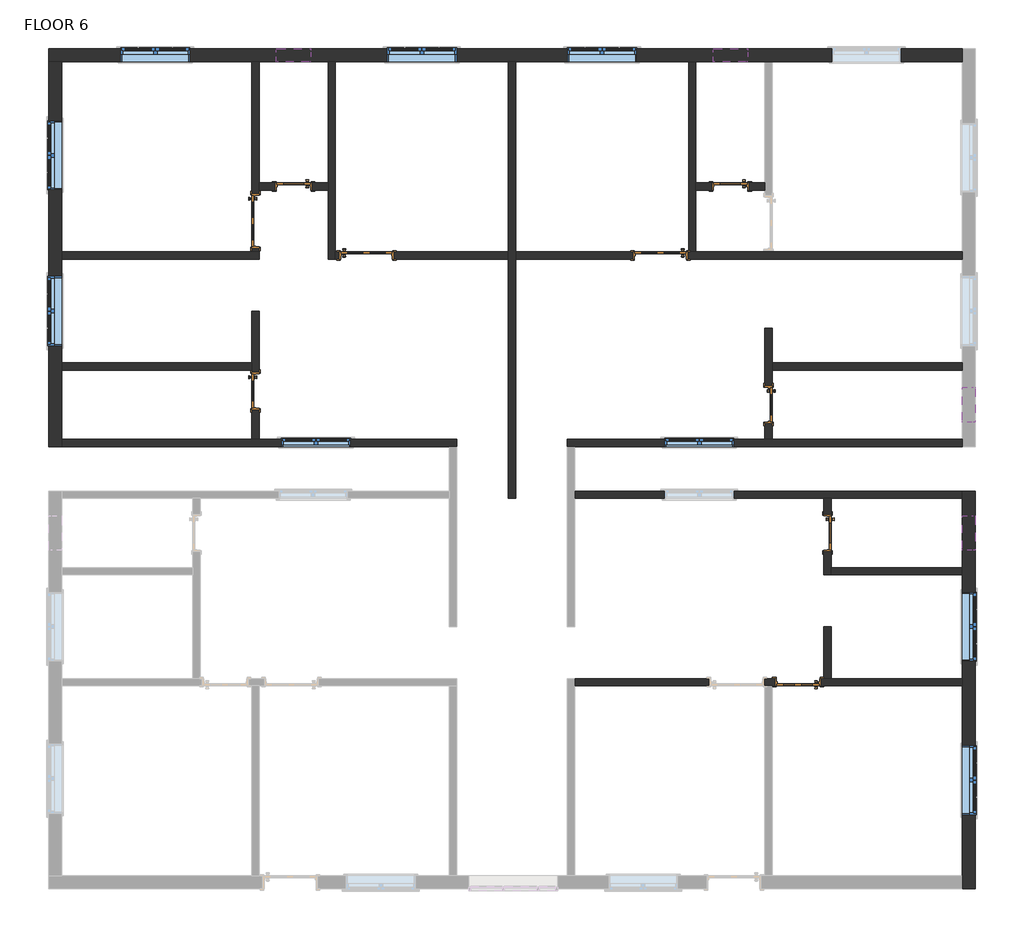
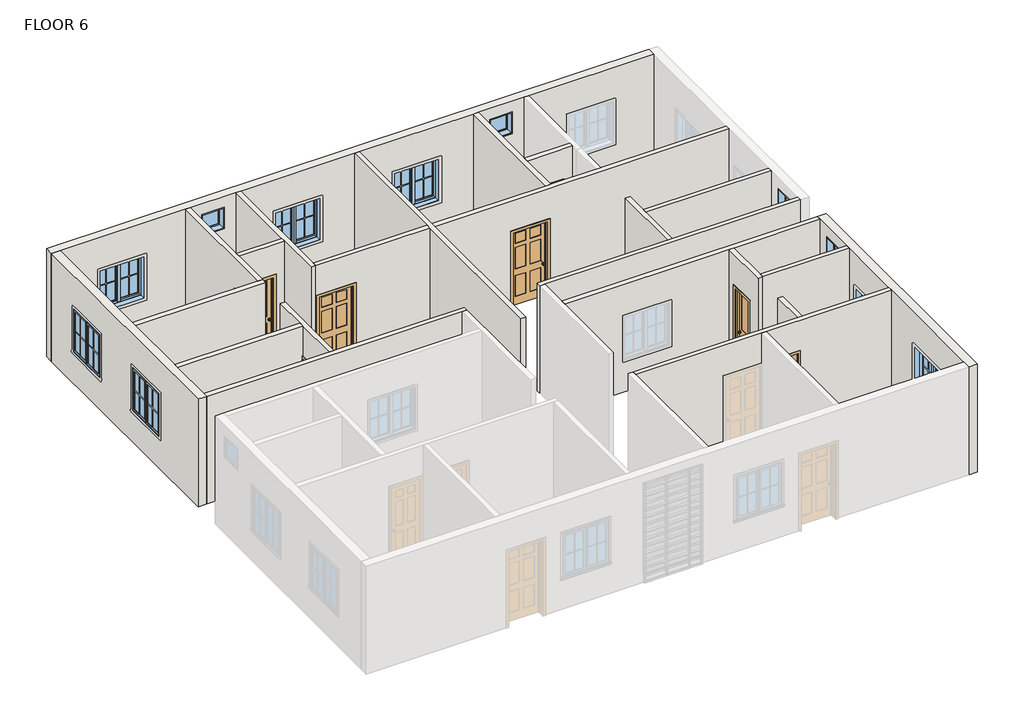
# One storey, part 3 of 4: 23 walls, 13 windows, 9 doors.
"""IFC4 building model written with IfcOpenShell, lengths in millimetres."""

from ifc_helpers import new_model, si_unit, frame, origin, place, context, project, spatial, polyline, outline, extrude, faceted_brep, transform, mapped, element, save
from components import door_e337afa5, door_596d7c92, door_d66ee888, door_c610b25b, door_03e3dfb5, window_80340324, window_9200f5ac, window_c2c97eee

model = new_model("IFC4")

# Units and contexts
model_context = context("Model", 3, world=origin())
ifc_project = project(units=[si_unit("LENGTHUNIT", "METRE", prefix="MILLI")], contexts=[model_context])

# Site, building, storey
site = spatial("IfcSite", under=ifc_project)
building = spatial("IfcBuilding", under=site)
storey = spatial("IfcBuildingStorey", under=building, Name="FLOOR 6", Elevation=9544.3725604)

# Doors
placement = place(None, origin())
door_shape = door_e337afa5(model_context)
element("IfcDoor", 1, ObjectType="Door-Interior-Single-2_Panel-Wood : 24\" x 84\"", at=placement, inside=storey, context=model_context, shape_type="MappedRepresentation", body=[
    mapped(door_shape, transform((-8112.4137331, 4563.2156164, 9544.3725604), x_axis=(-1.0, 0.0, 0.0), y_axis=(0.0, -1.0, 0.0), z_axis=(0.0, 0.0, 1.0))),
])
element("IfcDoor", 2, ObjectType="Door-Interior-Single-2_Panel-Wood : 24\" x 84\"", at=placement, inside=storey, context=model_context, shape_type="MappedRepresentation", body=[
    mapped(door_shape, transform((-416.2137331, 4563.2156164, 9544.3725604), x_axis=(-1.0, 0.0, 0.0), y_axis=(0.0, -1.0, 0.0), z_axis=(0.0, 0.0, 1.0))),
])
element("IfcDoor", 3, ObjectType="Door-Interior-Single-2_Panel-Wood : 24\" x 84\"", at=placement, inside=storey, context=model_context, shape_type="MappedRepresentation", body=[
    mapped(door_shape, transform((-8788.6887331, 953.2406164, 9544.3725604), x_axis=(0.0, -1.0, 0.0), y_axis=(1.0, 0.0, 0.0), z_axis=(0.0, 0.0, 1.0))),
])
door_2_shape = door_596d7c92(model_context)
element("IfcDoor", 4, ObjectType="Door-Interior-Single-2_Panel-Wood : 24\" x 84\"", at=placement, inside=storey, context=model_context, shape_type="MappedRepresentation", body=[
    mapped(door_2_shape, transform((260.0612669, 711.9406164, 9544.3725604), x_axis=(0.0, -1.0, 0.0), y_axis=(1.0, 0.0, 0.0), z_axis=(0.0, 0.0, 1.0))),
])
element("IfcDoor", 5, ObjectType="Door-Interior-Single-2_Panel-Wood : 24\" x 84\"", at=placement, inside=storey, context=model_context, shape_type="MappedRepresentation", body=[
    mapped(door_2_shape, transform((1301.4612669, -1548.6593836, 9544.3725604), x_axis=(0.0, -1.0, 0.0), y_axis=(1.0, 0.0, 0.0), z_axis=(0.0, 0.0, 1.0))),
])
door_3_shape = door_d66ee888(model_context)
element("IfcDoor", 6, ObjectType="Door-Interior-Single-6_Panel-Wood : 30\" x 84\"", at=placement, inside=storey, context=model_context, shape_type="MappedRepresentation", body=[
    mapped(door_3_shape, transform((777.5862669, -4180.7343836, 9544.3725604), x_axis=(-1.0, 0.0, 0.0), y_axis=(0.0, -1.0, 0.0), z_axis=(0.0, 0.0, 1.0))),
])
door_4_shape = door_c610b25b(model_context)
element("IfcDoor", 7, ObjectType="Door-Interior-Single-6_Panel-Wood : 36\" x 84\"", at=placement, inside=storey, context=model_context, shape_type="MappedRepresentation", body=[
    mapped(door_4_shape, transform((-8788.6887331, 3950.4406164, 9544.3725604), x_axis=(0.0, -1.0, 0.0), y_axis=(1.0, 0.0, 0.0), z_axis=(0.0, 0.0, 1.0))),
])
element("IfcDoor", 8, ObjectType="Door-Interior-Single-6_Panel-Wood : 36\" x 84\"", at=placement, inside=storey, context=model_context, shape_type="MappedRepresentation", body=[
    mapped(door_4_shape, transform((-1648.1137331, 3344.0156164, 9544.3725604), x_axis=(-1.0, 0.0, 0.0), y_axis=(0.0, -1.0, 0.0), z_axis=(0.0, 0.0, 1.0))),
])
door_5_shape = door_03e3dfb5(model_context)
element("IfcDoor", 9, ObjectType="Door-Interior-Single-6_Panel-Wood : 36\" x 84\"", at=placement, inside=storey, context=model_context, shape_type="MappedRepresentation", body=[
    mapped(door_5_shape, transform((-6829.7137331, 3344.0156164, 9544.3725604), x_axis=(1.0, 0.0, 0.0), y_axis=(0.0, 1.0, 0.0), z_axis=(0.0, 0.0, 1.0))),
])

# Walls
element("IfcWall", 10, ObjectType="Inner Wall 5\"", at=placement, inside=storey, context=model_context, shape_type="Brep", body=[
    faceted_brep([(-12201.8137331, -24.6593836, 9544.3725604), (-5369.2137331, -24.6593836, 9544.3725604), (-5242.2137331, -24.6593836, 9544.3725604), (-5242.2137331, -24.6593836, 12592.3725604), (-5369.2137331, -24.6593836, 12592.3725604), (-12201.8137331, -24.6593836, 12592.3725604), (-7109.1137331, -24.6593836, 11677.9725604), (-7109.1137331, -24.6593836, 10458.7725604), (-8328.3137331, -24.6593836, 10458.7725604), (-8328.3137331, -24.6593836, 11677.9725604), (-12201.8137331, 102.3406164, 9544.3725604), (-12201.8137331, 102.3406164, 12592.3725604), (-8849.0137331, 102.3406164, 12592.3725604), (-8722.0137331, 102.3406164, 12592.3725604), (-5242.2137331, 102.3406164, 12592.3725604), (-5242.2137331, 102.3406164, 9544.3725604), (-8722.0137331, 102.3406164, 9544.3725604), (-8849.0137331, 102.3406164, 9544.3725604), (-7109.1137331, 102.3406164, 11677.9725604), (-8328.3137331, 102.3406164, 11677.9725604), (-8328.3137331, 102.3406164, 10458.7725604), (-7109.1137331, 102.3406164, 10458.7725604)], [[[0, 1, 2, 3, 4, 5], [6, 7, 8, 9]], [[10, 11, 12, 13, 14, 15, 16, 17], [18, 19, 20, 21]], [[2, 1, 0, 10, 17, 16, 15]], [[5, 4, 3, 14, 13, 12, 11]], [[0, 5, 11, 10]], [[3, 2, 15, 14]], [[7, 6, 18, 21]], [[8, 7, 21, 20]], [[9, 8, 20, 19]], [[6, 9, 19, 18]]]),
])
element("IfcWall", 11, ObjectType="Inner Wall 5\"", at=placement, inside=storey, context=model_context, shape_type="Brep", body=[
    faceted_brep([(3673.1862669, 102.3406164, 9544.3725604), (320.3862669, 102.3406164, 9544.3725604), (193.3862669, 102.3406164, 9544.3725604), (-3286.4137331, 102.3406164, 9544.3725604), (-3286.4137331, 102.3406164, 12592.3725604), (193.3862669, 102.3406164, 12592.3725604), (320.3862669, 102.3406164, 12592.3725604), (3673.1862669, 102.3406164, 12592.3725604), (-352.7137331, 102.3406164, 11677.9725604), (-1571.9137331, 102.3406164, 11677.9725604), (-1571.9137331, 102.3406164, 10458.7725604), (-352.7137331, 102.3406164, 10458.7725604), (3673.1862669, -24.6593836, 9544.3725604), (3673.1862669, -24.6593836, 12592.3725604), (-3159.4137331, -24.6593836, 12592.3725604), (-3286.4137331, -24.6593836, 12592.3725604), (-3286.4137331, -24.6593836, 9544.3725604), (-3159.4137331, -24.6593836, 9544.3725604), (-352.7137331, -24.6593836, 11677.9725604), (-352.7137331, -24.6593836, 10458.7725604), (-1571.9137331, -24.6593836, 10458.7725604), (-1571.9137331, -24.6593836, 11677.9725604)], [[[0, 1, 2, 3, 4, 5, 6, 7], [8, 9, 10, 11]], [[12, 13, 14, 15, 16, 17], [18, 19, 20, 21]], [[3, 2, 1, 0, 12, 17, 16]], [[7, 6, 5, 4, 15, 14, 13]], [[0, 7, 13, 12]], [[4, 3, 16, 15]], [[19, 18, 8, 11]], [[20, 19, 11, 10]], [[21, 20, 10, 9]], [[18, 21, 9, 8]]]),
])
element("IfcWall", 12, ObjectType="Inner Wall 5\"", at=placement, inside=storey, context=model_context, shape_type="Brep", body=[
    faceted_brep([(3673.1862669, -812.0593836, 9544.3725604), (-3159.4137331, -812.0593836, 9544.3725604), (-3159.4137331, -812.0593836, 12592.3725604), (3673.1862669, -812.0593836, 12592.3725604), (-352.7137331, -812.0593836, 11677.9725604), (-1571.9137331, -812.0593836, 11677.9725604), (-1571.9137331, -812.0593836, 10458.7725604), (-352.7137331, -812.0593836, 10458.7725604), (3673.1862669, -939.0593836, 9544.3725604), (3673.1862669, -939.0593836, 12592.3725604), (1361.7862669, -939.0593836, 12592.3725604), (1234.7862669, -939.0593836, 12592.3725604), (-3159.4137331, -939.0593836, 12592.3725604), (-3159.4137331, -939.0593836, 9544.3725604), (1234.7862669, -939.0593836, 9544.3725604), (1361.7862669, -939.0593836, 9544.3725604), (-352.7137331, -939.0593836, 11677.9725604), (-352.7137331, -939.0593836, 10458.7725604), (-1571.9137331, -939.0593836, 10458.7725604), (-1571.9137331, -939.0593836, 11677.9725604)], [[[0, 1, 2, 3], [4, 5, 6, 7]], [[8, 9, 10, 11, 12, 13, 14, 15], [16, 17, 18, 19]], [[1, 0, 8, 15, 14, 13]], [[3, 2, 12, 11, 10, 9]], [[0, 3, 9, 8]], [[2, 1, 13, 12]], [[17, 16, 4, 7]], [[18, 17, 7, 6]], [[19, 18, 6, 5]], [[16, 19, 5, 4]]]),
])
element("IfcWall", 13, ObjectType="Inner Wall 5\"", at=placement, inside=storey, context=model_context, shape_type="Brep", body=[
    faceted_brep([(1234.7862669, -2285.2593836, 12592.3725604), (1234.7862669, -939.0593836, 12592.3725604), (1234.7862669, -939.0593836, 9544.3725604), (1234.7862669, -1218.4593836, 9544.3725604), (1234.7862669, -1218.4593836, 11703.3725604), (1234.7862669, -1878.8593836, 11703.3725604), (1234.7862669, -1878.8593836, 9544.3725604), (1234.7862669, -2285.2593836, 9544.3725604), (1361.7862669, -939.0593836, 12592.3725604), (1361.7862669, -2158.2593836, 12592.3725604), (1361.7862669, -2285.2593836, 12592.3725604), (1361.7862669, -2285.2593836, 9544.3725604), (1361.7862669, -2158.2593836, 9544.3725604), (1361.7862669, -1878.8593836, 9544.3725604), (1361.7862669, -1878.8593836, 11703.3725604), (1361.7862669, -1218.4593836, 11703.3725604), (1361.7862669, -1218.4593836, 9544.3725604), (1361.7862669, -939.0593836, 9544.3725604)], [[[0, 1, 2, 3, 4, 5, 6, 7]], [[8, 9, 10, 11, 12, 13, 14, 15, 16, 17]], [[2, 17, 16, 3]], [[11, 7, 6, 13, 12]], [[1, 0, 10, 9, 8]], [[2, 1, 8, 17]], [[0, 7, 11, 10]], [[5, 14, 13, 6]], [[14, 5, 4, 15]], [[15, 4, 3, 16]]]),
])
element("IfcWall", 14, ObjectType="Inner Wall 5\"", at=placement, inside=storey, context=model_context, shape_type="SweptSolid", body=[
    extrude(outline(polyline([(3673.1862669, -2285.2593836), (1361.7862669, -2285.2593836), (1361.7862669, -2158.2593836), (3673.1862669, -2158.2593836), (3673.1862669, -2285.2593836)])), frame((0.0, 0.0, 9544.3725604), z_axis=(0.0, 0.0, 1.0), x_axis=(1.0, 0.0, 0.0)), (0.0, 0.0, 1.0), 3048.0),
])
element("IfcWall", 15, ObjectType="Inner Wall 5\"", at=placement, inside=storey, context=model_context, shape_type="Brep", body=[
    faceted_brep([(3673.1862669, -4241.0593836, 12592.3725604), (320.3862669, -4241.0593836, 12592.3725604), (193.3862669, -4241.0593836, 12592.3725604), (-3159.4137331, -4241.0593836, 12592.3725604), (-3159.4137331, -4241.0593836, 9544.3725604), (-784.5137331, -4241.0593836, 9544.3725604), (-784.5137331, -4241.0593836, 11703.3725604), (180.6862669, -4241.0593836, 11703.3725604), (180.6862669, -4241.0593836, 9544.3725604), (193.3862669, -4241.0593836, 9544.3725604), (320.3862669, -4241.0593836, 9544.3725604), (371.1862669, -4241.0593836, 9544.3725604), (371.1862669, -4241.0593836, 11703.3725604), (1183.9862669, -4241.0593836, 11703.3725604), (1183.9862669, -4241.0593836, 9544.3725604), (3673.1862669, -4241.0593836, 9544.3725604), (-3159.4137331, -4114.0593836, 12592.3725604), (1234.7862669, -4114.0593836, 12592.3725604), (1361.7862669, -4114.0593836, 12592.3725604), (3673.1862669, -4114.0593836, 12592.3725604), (3673.1862669, -4114.0593836, 9544.3725604), (1361.7862669, -4114.0593836, 9544.3725604), (1234.7862669, -4114.0593836, 9544.3725604), (1183.9862669, -4114.0593836, 9544.3725604), (1183.9862669, -4114.0593836, 11703.3725604), (371.1862669, -4114.0593836, 11703.3725604), (371.1862669, -4114.0593836, 9544.3725604), (180.6862669, -4114.0593836, 9544.3725604), (180.6862669, -4114.0593836, 11703.3725604), (-784.5137331, -4114.0593836, 11703.3725604), (-784.5137331, -4114.0593836, 9544.3725604), (-3159.4137331, -4114.0593836, 9544.3725604)], [[[0, 1, 2, 3, 4, 5, 6, 7, 8, 9, 10, 11, 12, 13, 14, 15]], [[16, 17, 18, 19, 20, 21, 22, 23, 24, 25, 26, 27, 28, 29, 30, 31]], [[4, 31, 30, 5]], [[20, 15, 14, 23, 22, 21]], [[8, 27, 26, 11, 10, 9]], [[3, 2, 1, 0, 19, 18, 17, 16]], [[4, 3, 16, 31]], [[0, 15, 20, 19]], [[7, 28, 27, 8]], [[28, 7, 6, 29]], [[29, 6, 5, 30]], [[25, 12, 11, 26]], [[12, 25, 24, 13]], [[13, 24, 23, 14]]]),
])
element("IfcWall", 16, ObjectType="Inner Wall 5\"", at=placement, inside=storey, context=model_context, shape_type="SweptSolid", body=[
    extrude(outline(polyline([(1361.7862669, -3199.6593836), (1361.7862669, -4114.0593836), (1234.7862669, -4114.0593836), (1234.7862669, -3199.6593836), (1361.7862669, -3199.6593836)])), frame((0.0, 0.0, 9544.3725604), z_axis=(0.0, 0.0, 1.0), x_axis=(1.0, 0.0, 0.0)), (0.0, 0.0, 1.0), 3048.0),
])
element("IfcWall", 17, ObjectType="Inner Wall 5\"", at=placement, inside=storey, context=model_context, shape_type="Brep", body=[
    faceted_brep([(-12201.8137331, 3277.3406164, 9544.3725604), (-8722.0137331, 3277.3406164, 9544.3725604), (-8722.0137331, 3277.3406164, 12592.3725604), (-12201.8137331, 3277.3406164, 12592.3725604), (-12201.8137331, 3404.3406164, 9544.3725604), (-12201.8137331, 3404.3406164, 12592.3725604), (-8849.0137331, 3404.3406164, 12592.3725604), (-8722.0137331, 3404.3406164, 12592.3725604), (-8722.0137331, 3404.3406164, 9544.3725604), (-8849.0137331, 3404.3406164, 9544.3725604)], [[[0, 1, 2, 3]], [[4, 5, 6, 7, 8, 9]], [[1, 0, 4, 9, 8]], [[3, 2, 7, 6, 5]], [[0, 3, 5, 4]], [[2, 1, 8, 7]]]),
])
element("IfcWall", 18, ObjectType="Inner Wall 5\"", at=placement, inside=storey, context=model_context, shape_type="Brep", body=[
    faceted_brep([(-8722.0137331, 6758.7281164, 12592.3725604), (-8722.0137331, 4623.5406164, 12592.3725604), (-8722.0137331, 4496.5406164, 12592.3725604), (-8722.0137331, 3404.3406164, 12592.3725604), (-8722.0137331, 3404.3406164, 9544.3725604), (-8722.0137331, 3467.8406164, 9544.3725604), (-8722.0137331, 3467.8406164, 11703.3725604), (-8722.0137331, 4433.0406164, 11703.3725604), (-8722.0137331, 4433.0406164, 9544.3725604), (-8722.0137331, 4496.5406164, 9544.3725604), (-8722.0137331, 4623.5406164, 9544.3725604), (-8722.0137331, 6758.7281164, 9544.3725604), (-8849.0137331, 3404.3406164, 12592.3725604), (-8849.0137331, 6758.7281164, 12592.3725604), (-8849.0137331, 6758.7281164, 9544.3725604), (-8849.0137331, 4433.0406164, 9544.3725604), (-8849.0137331, 4433.0406164, 11703.3725604), (-8849.0137331, 3467.8406164, 11703.3725604), (-8849.0137331, 3467.8406164, 9544.3725604), (-8849.0137331, 3404.3406164, 9544.3725604)], [[[0, 1, 2, 3, 4, 5, 6, 7, 8, 9, 10, 11]], [[12, 13, 14, 15, 16, 17, 18, 19]], [[4, 19, 18, 5]], [[14, 11, 10, 9, 8, 15]], [[3, 2, 1, 0, 13, 12]], [[4, 3, 12, 19]], [[0, 11, 14, 13]], [[17, 6, 5, 18]], [[6, 17, 16, 7]], [[7, 16, 15, 8]]]),
])
element("IfcWall", 19, ObjectType="Inner Wall 5\"", at=placement, inside=storey, context=model_context, shape_type="SweptSolid", body=[
    extrude(outline(polyline([(12592.3725604, -7502.8137331), (12592.3725604, -8722.0137331), (9544.3725604, -8722.0137331), (9544.3725604, -8442.6137331), (11703.3725604, -8442.6137331), (11703.3725604, -7782.2137331), (9544.3725604, -7782.2137331), (9544.3725604, -7502.8137331), (12592.3725604, -7502.8137331)])), frame((0.0, 4496.5406164, 0.0), z_axis=(0.0, 1.0, 0.0), x_axis=(0.0, 0.0, 1.0)), (0.0, 0.0, 1.0), 127.0),
])
element("IfcWall", 20, ObjectType="Inner Wall 5\"", at=placement, inside=storey, context=model_context, shape_type="Brep", body=[
    faceted_brep([(-7375.8137331, 3277.3406164, 9544.3725604), (-7375.8137331, 3404.3406164, 9544.3725604), (-7375.8137331, 6758.7281164, 9544.3725604), (-7375.8137331, 6758.7281164, 12592.3725604), (-7375.8137331, 3404.3406164, 12592.3725604), (-7375.8137331, 3277.3406164, 12592.3725604), (-7502.8137331, 3277.3406164, 9544.3725604), (-7502.8137331, 3277.3406164, 12592.3725604), (-7502.8137331, 4496.5406164, 12592.3725604), (-7502.8137331, 4623.5406164, 12592.3725604), (-7502.8137331, 6758.7281164, 12592.3725604), (-7502.8137331, 6758.7281164, 9544.3725604), (-7502.8137331, 4623.5406164, 9544.3725604), (-7502.8137331, 4496.5406164, 9544.3725604)], [[[0, 1, 2, 3, 4, 5]], [[6, 7, 8, 9, 10, 11, 12, 13]], [[2, 1, 0, 6, 13, 12, 11]], [[5, 4, 3, 10, 9, 8, 7]], [[3, 2, 11, 10]], [[0, 5, 7, 6]]]),
])
element("IfcWall", 21, ObjectType="Inner Wall 5\"", at=placement, inside=storey, context=model_context, shape_type="Brep", body=[
    faceted_brep([(-4327.8137331, 6758.7281164, 9544.3725604), (-4327.8137331, 3404.3406164, 9544.3725604), (-4327.8137331, 3277.3406164, 9544.3725604), (-4327.8137331, -939.0593836, 9544.3725604), (-4327.8137331, -939.0593836, 12592.3725604), (-4327.8137331, 3277.3406164, 12592.3725604), (-4327.8137331, 3404.3406164, 12592.3725604), (-4327.8137331, 6758.7281164, 12592.3725604), (-4200.8137331, 6758.7281164, 9544.3725604), (-4200.8137331, 6758.7281164, 12592.3725604), (-4200.8137331, 3404.3406164, 12592.3725604), (-4200.8137331, 3277.3406164, 12592.3725604), (-4200.8137331, -939.0593836, 12592.3725604), (-4200.8137331, -939.0593836, 9544.3725604), (-4200.8137331, 3277.3406164, 9544.3725604), (-4200.8137331, 3404.3406164, 9544.3725604)], [[[0, 1, 2, 3, 4, 5, 6, 7]], [[8, 9, 10, 11, 12, 13, 14, 15]], [[3, 2, 1, 0, 8, 15, 14, 13]], [[4, 3, 13, 12]], [[7, 6, 5, 4, 12, 11, 10, 9]], [[0, 7, 9, 8]]]),
])
element("IfcWall", 22, ObjectType="Inner Wall 5\"", at=placement, inside=storey, context=model_context, shape_type="SweptSolid", body=[
    extrude(outline(polyline([(12592.3725604, -4327.8137331), (12592.3725604, -7375.8137331), (9544.3725604, -7375.8137331), (9544.3725604, -7312.3137331), (11703.3725604, -7312.3137331), (11703.3725604, -6347.1137331), (9544.3725604, -6347.1137331), (9544.3725604, -4327.8137331), (12592.3725604, -4327.8137331)])), frame((0.0, 3277.3406164, 0.0), z_axis=(0.0, 1.0, 0.0), x_axis=(0.0, 0.0, 1.0)), (0.0, 0.0, 1.0), 127.0),
])
element("IfcWall", 23, ObjectType="Inner Wall 5\"", at=placement, inside=storey, context=model_context, shape_type="Brep", body=[
    faceted_brep([(3673.1862669, 3277.3406164, 12592.3725604), (-4200.8137331, 3277.3406164, 12592.3725604), (-4200.8137331, 3277.3406164, 9544.3725604), (-2130.7137331, 3277.3406164, 9544.3725604), (-2130.7137331, 3277.3406164, 11703.3725604), (-1165.5137331, 3277.3406164, 11703.3725604), (-1165.5137331, 3277.3406164, 9544.3725604), (3673.1862669, 3277.3406164, 9544.3725604), (-4200.8137331, 3404.3406164, 12592.3725604), (-1152.8137331, 3404.3406164, 12592.3725604), (-1025.8137331, 3404.3406164, 12592.3725604), (193.3862669, 3404.3406164, 12592.3725604), (320.3862669, 3404.3406164, 12592.3725604), (3673.1862669, 3404.3406164, 12592.3725604), (3673.1862669, 3404.3406164, 9544.3725604), (320.3862669, 3404.3406164, 9544.3725604), (193.3862669, 3404.3406164, 9544.3725604), (-1025.8137331, 3404.3406164, 9544.3725604), (-1152.8137331, 3404.3406164, 9544.3725604), (-1165.5137331, 3404.3406164, 9544.3725604), (-1165.5137331, 3404.3406164, 11703.3725604), (-2130.7137331, 3404.3406164, 11703.3725604), (-2130.7137331, 3404.3406164, 9544.3725604), (-4200.8137331, 3404.3406164, 9544.3725604)], [[[0, 1, 2, 3, 4, 5, 6, 7]], [[8, 9, 10, 11, 12, 13, 14, 15, 16, 17, 18, 19, 20, 21, 22, 23]], [[2, 23, 22, 3]], [[14, 7, 6, 19, 18, 17, 16, 15]], [[1, 0, 13, 12, 11, 10, 9, 8]], [[2, 1, 8, 23]], [[0, 7, 14, 13]], [[21, 4, 3, 22]], [[4, 21, 20, 5]], [[5, 20, 19, 6]]]),
])
element("IfcWall", 24, ObjectType="Inner Wall 5\"", at=placement, inside=storey, context=model_context, shape_type="Brep", body=[
    faceted_brep([(-1025.8137331, 3404.3406164, 9544.3725604), (-1025.8137331, 4496.5406164, 9544.3725604), (-1025.8137331, 4623.5406164, 9544.3725604), (-1025.8137331, 6758.7281164, 9544.3725604), (-1025.8137331, 6758.7281164, 12592.3725604), (-1025.8137331, 4623.5406164, 12592.3725604), (-1025.8137331, 4496.5406164, 12592.3725604), (-1025.8137331, 3404.3406164, 12592.3725604), (-1152.8137331, 3404.3406164, 9544.3725604), (-1152.8137331, 3404.3406164, 12592.3725604), (-1152.8137331, 6758.7281164, 12592.3725604), (-1152.8137331, 6758.7281164, 9544.3725604)], [[[0, 1, 2, 3, 4, 5, 6, 7]], [[8, 9, 10, 11]], [[3, 2, 1, 0, 8, 11]], [[7, 6, 5, 4, 10, 9]], [[0, 7, 9, 8]], [[4, 3, 11, 10]]]),
])
element("IfcWall", 25, ObjectType="Inner Wall 5\"", at=placement, inside=storey, context=model_context, shape_type="SweptSolid", body=[
    extrude(outline(polyline([(12592.3725604, 193.3862669), (12592.3725604, -1025.8137331), (9544.3725604, -1025.8137331), (9544.3725604, -746.4137331), (11703.3725604, -746.4137331), (11703.3725604, -86.0137331), (9544.3725604, -86.0137331), (9544.3725604, 193.3862669), (12592.3725604, 193.3862669)])), frame((0.0, 4496.5406164, 0.0), z_axis=(0.0, 1.0, 0.0), x_axis=(0.0, 0.0, 1.0)), (0.0, 0.0, 1.0), 127.0),
])
element("IfcWall", 26, ObjectType="Inner Wall 5\"", at=placement, inside=storey, context=model_context, shape_type="SweptSolid", body=[
    extrude(outline(polyline([(320.3862669, 1448.5406164), (3673.1862669, 1448.5406164), (3673.1862669, 1321.5406164), (320.3862669, 1321.5406164), (320.3862669, 1448.5406164)])), frame((0.0, 0.0, 9544.3725604), z_axis=(0.0, 0.0, 1.0), x_axis=(1.0, 0.0, 0.0)), (0.0, 0.0, 1.0), 3048.0),
])
element("IfcWall", 27, ObjectType="Inner Wall 5\"", at=placement, inside=storey, context=model_context, shape_type="Brep", body=[
    faceted_brep([(193.3862669, 102.3406164, 12592.3725604), (193.3862669, 2058.1406164, 12592.3725604), (193.3862669, 2058.1406164, 9544.3725604), (193.3862669, 1042.1406164, 9544.3725604), (193.3862669, 1042.1406164, 11703.3725604), (193.3862669, 381.7406164, 11703.3725604), (193.3862669, 381.7406164, 9544.3725604), (193.3862669, 102.3406164, 9544.3725604), (320.3862669, 2058.1406164, 12592.3725604), (320.3862669, 1448.5406164, 12592.3725604), (320.3862669, 1321.5406164, 12592.3725604), (320.3862669, 102.3406164, 12592.3725604), (320.3862669, 102.3406164, 9544.3725604), (320.3862669, 381.7406164, 9544.3725604), (320.3862669, 381.7406164, 11703.3725604), (320.3862669, 1042.1406164, 11703.3725604), (320.3862669, 1042.1406164, 9544.3725604), (320.3862669, 1321.5406164, 9544.3725604), (320.3862669, 1448.5406164, 9544.3725604), (320.3862669, 2058.1406164, 9544.3725604)], [[[0, 1, 2, 3, 4, 5, 6, 7]], [[8, 9, 10, 11, 12, 13, 14, 15, 16, 17, 18, 19]], [[2, 19, 18, 17, 16, 3]], [[12, 7, 6, 13]], [[1, 0, 11, 10, 9, 8]], [[2, 1, 8, 19]], [[0, 7, 12, 11]], [[5, 14, 13, 6]], [[14, 5, 4, 15]], [[15, 4, 3, 16]]]),
])
element("IfcWall", 28, ObjectType="Inner Wall 5\"", at=placement, inside=storey, context=model_context, shape_type="Brep", body=[
    faceted_brep([(-8722.0137331, 2362.9406164, 9544.3725604), (-8722.0137331, 2362.9406164, 12592.3725604), (-8722.0137331, 102.3406164, 12592.3725604), (-8722.0137331, 102.3406164, 9544.3725604), (-8722.0137331, 623.0406164, 9544.3725604), (-8722.0137331, 623.0406164, 11703.3725604), (-8722.0137331, 1283.4406164, 11703.3725604), (-8722.0137331, 1283.4406164, 9544.3725604), (-8849.0137331, 2362.9406164, 12592.3725604), (-8849.0137331, 2362.9406164, 9544.3725604), (-8849.0137331, 1448.5406164, 9544.3725604), (-8849.0137331, 1321.5406164, 9544.3725604), (-8849.0137331, 1283.4406164, 9544.3725604), (-8849.0137331, 1283.4406164, 11703.3725604), (-8849.0137331, 623.0406164, 11703.3725604), (-8849.0137331, 623.0406164, 9544.3725604), (-8849.0137331, 102.3406164, 9544.3725604), (-8849.0137331, 102.3406164, 12592.3725604), (-8849.0137331, 1321.5406164, 12592.3725604), (-8849.0137331, 1448.5406164, 12592.3725604)], [[[0, 1, 2, 3, 4, 5, 6, 7]], [[8, 9, 10, 11, 12, 13, 14, 15, 16, 17, 18, 19]], [[9, 0, 7, 12, 11, 10]], [[3, 16, 15, 4]], [[1, 0, 9, 8]], [[2, 1, 8, 19, 18, 17]], [[3, 2, 17, 16]], [[14, 5, 4, 15]], [[5, 14, 13, 6]], [[6, 13, 12, 7]]]),
])
element("IfcWall", 29, ObjectType="Inner Wall 5\"", at=placement, inside=storey, context=model_context, shape_type="SweptSolid", body=[
    extrude(outline(polyline([(-12201.8137331, 1448.5406164), (-8849.0137331, 1448.5406164), (-8849.0137331, 1321.5406164), (-12201.8137331, 1321.5406164), (-12201.8137331, 1448.5406164)])), frame((0.0, 0.0, 9544.3725604), z_axis=(0.0, 0.0, 1.0), x_axis=(1.0, 0.0, 0.0)), (0.0, 0.0, 1.0), 3048.0),
])
element("IfcWall", 30, ObjectType="outer wall 9\"", at=placement, inside=storey, context=model_context, shape_type="Brep", body=[
    faceted_brep([(-12430.4137331, 6758.7281164, 9544.3725604), (-12201.8137331, 6758.7281164, 9544.3725604), (-8849.0137331, 6758.7281164, 9544.3725604), (-8722.0137331, 6758.7281164, 9544.3725604), (-7502.8137331, 6758.7281164, 9544.3725604), (-7375.8137331, 6758.7281164, 9544.3725604), (-4327.8137331, 6758.7281164, 9544.3725604), (-4200.8137331, 6758.7281164, 9544.3725604), (-1152.8137331, 6758.7281164, 9544.3725604), (-1025.8137331, 6758.7281164, 9544.3725604), (193.3862669, 6758.7281164, 9544.3725604), (320.3862669, 6758.7281164, 9544.3725604), (3673.1862669, 6758.7281164, 9544.3725604), (3673.1862669, 6758.7281164, 12592.3725604), (320.3862669, 6758.7281164, 12592.3725604), (193.3862669, 6758.7281164, 12592.3725604), (-1025.8137331, 6758.7281164, 12592.3725604), (-1152.8137331, 6758.7281164, 12592.3725604), (-4200.8137331, 6758.7281164, 12592.3725604), (-4327.8137331, 6758.7281164, 12592.3725604), (-7375.8137331, 6758.7281164, 12592.3725604), (-7502.8137331, 6758.7281164, 12592.3725604), (-8722.0137331, 6758.7281164, 12592.3725604), (-8849.0137331, 6758.7281164, 12592.3725604), (-12201.8137331, 6758.7281164, 12592.3725604), (-12430.4137331, 6758.7281164, 12592.3725604), (-9941.2137331, 6758.7281164, 11677.9725604), (-9941.2137331, 6758.7281164, 10458.7725604), (-11160.4137331, 6758.7281164, 10458.7725604), (-11160.4137331, 6758.7281164, 11677.9725604), (-5242.2137331, 6758.7281164, 11677.9725604), (-5242.2137331, 6758.7281164, 10458.7725604), (-6461.4137331, 6758.7281164, 10458.7725604), (-6461.4137331, 6758.7281164, 11677.9725604), (-2067.2137331, 6758.7281164, 11677.9725604), (-2067.2137331, 6758.7281164, 10458.7725604), (-3286.4137331, 6758.7281164, 10458.7725604), (-3286.4137331, 6758.7281164, 11677.9725604), (2593.6862669, 6758.7281164, 11677.9725604), (2593.6862669, 6758.7281164, 10458.7725604), (1374.4862669, 6758.7281164, 10458.7725604), (1374.4862669, 6758.7281164, 11677.9725604), (-7807.6137331, 6758.7281164, 12287.5725604), (-7807.6137331, 6758.7281164, 11677.9725604), (-8417.2137331, 6758.7281164, 11677.9725604), (-8417.2137331, 6758.7281164, 12287.5725604), (-111.4137331, 6758.7281164, 12287.5725604), (-111.4137331, 6758.7281164, 11677.9725604), (-721.0137331, 6758.7281164, 11677.9725604), (-721.0137331, 6758.7281164, 12287.5725604), (-12430.4137331, 6987.3281164, 9544.3725604), (-12430.4137331, 6987.3281164, 12592.3725604), (3673.1862669, 6987.3281164, 12592.3725604), (3673.1862669, 6987.3281164, 9544.3725604), (-9941.2137331, 6987.3281164, 11677.9725604), (-11160.4137331, 6987.3281164, 11677.9725604), (-11160.4137331, 6987.3281164, 10458.7725604), (-9941.2137331, 6987.3281164, 10458.7725604), (-5242.2137331, 6987.3281164, 11677.9725604), (-6461.4137331, 6987.3281164, 11677.9725604), (-6461.4137331, 6987.3281164, 10458.7725604), (-5242.2137331, 6987.3281164, 10458.7725604), (-2067.2137331, 6987.3281164, 11677.9725604), (-3286.4137331, 6987.3281164, 11677.9725604), (-3286.4137331, 6987.3281164, 10458.7725604), (-2067.2137331, 6987.3281164, 10458.7725604), (2593.6862669, 6987.3281164, 11677.9725604), (1374.4862669, 6987.3281164, 11677.9725604), (1374.4862669, 6987.3281164, 10458.7725604), (2593.6862669, 6987.3281164, 10458.7725604), (-7807.6137331, 6987.3281164, 12287.5725604), (-8417.2137331, 6987.3281164, 12287.5725604), (-8417.2137331, 6987.3281164, 11677.9725604), (-7807.6137331, 6987.3281164, 11677.9725604), (-111.4137331, 6987.3281164, 12287.5725604), (-721.0137331, 6987.3281164, 12287.5725604), (-721.0137331, 6987.3281164, 11677.9725604), (-111.4137331, 6987.3281164, 11677.9725604)], [[[0, 1, 2, 3, 4, 5, 6, 7, 8, 9, 10, 11, 12, 13, 14, 15, 16, 17, 18, 19, 20, 21, 22, 23, 24, 25], [26, 27, 28, 29], [30, 31, 32, 33], [34, 35, 36, 37], [38, 39, 40, 41], [42, 43, 44, 45], [46, 47, 48, 49]], [[50, 51, 52, 53], [54, 55, 56, 57], [58, 59, 60, 61], [62, 63, 64, 65], [66, 67, 68, 69], [70, 71, 72, 73], [74, 75, 76, 77]], [[12, 11, 10, 9, 8, 7, 6, 5, 4, 3, 2, 1, 0, 50, 53]], [[25, 24, 23, 22, 21, 20, 19, 18, 17, 16, 15, 14, 13, 52, 51]], [[0, 25, 51, 50]], [[13, 12, 53, 52]], [[27, 26, 54, 57]], [[28, 27, 57, 56]], [[29, 28, 56, 55]], [[26, 29, 55, 54]], [[31, 30, 58, 61]], [[32, 31, 61, 60]], [[33, 32, 60, 59]], [[30, 33, 59, 58]], [[35, 34, 62, 65]], [[36, 35, 65, 64]], [[37, 36, 64, 63]], [[34, 37, 63, 62]], [[39, 38, 66, 69]], [[40, 39, 69, 68]], [[41, 40, 68, 67]], [[38, 41, 67, 66]], [[43, 42, 70, 73]], [[44, 43, 73, 72]], [[45, 44, 72, 71]], [[42, 45, 71, 70]], [[47, 46, 74, 77]], [[48, 47, 77, 76]], [[49, 48, 76, 75]], [[46, 49, 75, 74]]]),
])
element("IfcWall", 31, ObjectType="outer wall 9\"", at=placement, inside=storey, context=model_context, shape_type="Brep", body=[
    faceted_brep([(-12201.8137331, -24.6593836, 9544.3725604), (-12201.8137331, 102.3406164, 9544.3725604), (-12201.8137331, 1321.5406164, 9544.3725604), (-12201.8137331, 1448.5406164, 9544.3725604), (-12201.8137331, 3277.3406164, 9544.3725604), (-12201.8137331, 3404.3406164, 9544.3725604), (-12201.8137331, 6758.7281164, 9544.3725604), (-12201.8137331, 6758.7281164, 12592.3725604), (-12201.8137331, 3404.3406164, 12592.3725604), (-12201.8137331, 3277.3406164, 12592.3725604), (-12201.8137331, 1448.5406164, 12592.3725604), (-12201.8137331, 1321.5406164, 12592.3725604), (-12201.8137331, 102.3406164, 12592.3725604), (-12201.8137331, -24.6593836, 12592.3725604), (-12201.8137331, 2972.5406164, 11677.9725604), (-12201.8137331, 2972.5406164, 10458.7725604), (-12201.8137331, 1753.3406164, 10458.7725604), (-12201.8137331, 1753.3406164, 11677.9725604), (-12201.8137331, 5716.5343664, 11677.9725604), (-12201.8137331, 5716.5343664, 10458.7725604), (-12201.8137331, 4497.3343664, 10458.7725604), (-12201.8137331, 4497.3343664, 11677.9725604), (-12430.4137331, -24.6593836, 9544.3725604), (-12430.4137331, -24.6593836, 12592.3725604), (-12430.4137331, 6758.7281164, 12592.3725604), (-12430.4137331, 6758.7281164, 9544.3725604), (-12430.4137331, 2972.5406164, 11677.9725604), (-12430.4137331, 1753.3406164, 11677.9725604), (-12430.4137331, 1753.3406164, 10458.7725604), (-12430.4137331, 2972.5406164, 10458.7725604), (-12430.4137331, 5716.5343664, 11677.9725604), (-12430.4137331, 4497.3343664, 11677.9725604), (-12430.4137331, 4497.3343664, 10458.7725604), (-12430.4137331, 5716.5343664, 10458.7725604)], [[[0, 1, 2, 3, 4, 5, 6, 7, 8, 9, 10, 11, 12, 13], [14, 15, 16, 17], [18, 19, 20, 21]], [[22, 23, 24, 25], [26, 27, 28, 29], [30, 31, 32, 33]], [[6, 5, 4, 3, 2, 1, 0, 22, 25]], [[13, 12, 11, 10, 9, 8, 7, 24, 23]], [[7, 6, 25, 24]], [[0, 13, 23, 22]], [[15, 14, 26, 29]], [[16, 15, 29, 28]], [[17, 16, 28, 27]], [[14, 17, 27, 26]], [[19, 18, 30, 33]], [[20, 19, 33, 32]], [[21, 20, 32, 31]], [[18, 21, 31, 30]]]),
])
element("IfcWall", 32, ObjectType="outer wall 9\"", at=placement, inside=storey, context=model_context, shape_type="Brep", body=[
    faceted_brep([(3901.7862669, -7822.4593836, 9544.3725604), (3901.7862669, -812.0593836, 9544.3725604), (3901.7862669, -812.0593836, 12592.3725604), (3901.7862669, -7822.4593836, 12592.3725604), (3901.7862669, -3809.2593836, 11677.9725604), (3901.7862669, -2590.0593836, 11677.9725604), (3901.7862669, -2590.0593836, 10458.7725604), (3901.7862669, -3809.2593836, 10458.7725604), (3901.7862669, -6514.3593836, 11677.9725604), (3901.7862669, -5295.1593836, 11677.9725604), (3901.7862669, -5295.1593836, 10458.7725604), (3901.7862669, -6514.3593836, 10458.7725604), (3901.7862669, -1853.4593836, 12287.5725604), (3901.7862669, -1243.8593836, 12287.5725604), (3901.7862669, -1243.8593836, 11677.9725604), (3901.7862669, -1853.4593836, 11677.9725604), (3673.1862669, -7822.4593836, 9544.3725604), (3673.1862669, -7822.4593836, 12592.3725604), (3673.1862669, -7593.8593836, 12592.3725604), (3673.1862669, -4241.0593836, 12592.3725604), (3673.1862669, -4114.0593836, 12592.3725604), (3673.1862669, -2285.2593836, 12592.3725604), (3673.1862669, -2158.2593836, 12592.3725604), (3673.1862669, -939.0593836, 12592.3725604), (3673.1862669, -812.0593836, 12592.3725604), (3673.1862669, -812.0593836, 9544.3725604), (3673.1862669, -939.0593836, 9544.3725604), (3673.1862669, -2158.2593836, 9544.3725604), (3673.1862669, -2285.2593836, 9544.3725604), (3673.1862669, -4114.0593836, 9544.3725604), (3673.1862669, -4241.0593836, 9544.3725604), (3673.1862669, -7593.8593836, 9544.3725604), (3673.1862669, -3809.2593836, 11677.9725604), (3673.1862669, -3809.2593836, 10458.7725604), (3673.1862669, -2590.0593836, 10458.7725604), (3673.1862669, -2590.0593836, 11677.9725604), (3673.1862669, -6514.3593836, 11677.9725604), (3673.1862669, -6514.3593836, 10458.7725604), (3673.1862669, -5295.1593836, 10458.7725604), (3673.1862669, -5295.1593836, 11677.9725604), (3673.1862669, -1853.4593836, 12287.5725604), (3673.1862669, -1853.4593836, 11677.9725604), (3673.1862669, -1243.8593836, 11677.9725604), (3673.1862669, -1243.8593836, 12287.5725604)], [[[0, 1, 2, 3], [4, 5, 6, 7], [8, 9, 10, 11], [12, 13, 14, 15]], [[16, 17, 18, 19, 20, 21, 22, 23, 24, 25, 26, 27, 28, 29, 30, 31], [32, 33, 34, 35], [36, 37, 38, 39], [40, 41, 42, 43]], [[1, 0, 16, 31, 30, 29, 28, 27, 26, 25]], [[3, 2, 24, 23, 22, 21, 20, 19, 18, 17]], [[0, 3, 17, 16]], [[2, 1, 25, 24]], [[33, 32, 4, 7]], [[34, 33, 7, 6]], [[35, 34, 6, 5]], [[32, 35, 5, 4]], [[37, 36, 8, 11]], [[38, 37, 11, 10]], [[39, 38, 10, 9]], [[36, 39, 9, 8]], [[41, 40, 12, 15]], [[42, 41, 15, 14]], [[43, 42, 14, 13]], [[40, 43, 13, 12]]]),
])

# Windows
window_shape = window_80340324(model_context)
element("IfcWindow", 33, ObjectType="Fixed : 24\" x 24\"", at=placement, inside=storey, context=model_context, shape_type="MappedRepresentation", body=[
    mapped(window_shape, transform((3787.4862669, -1586.7593836, 10763.5725604), x_axis=(0.0, -1.0, 0.0), y_axis=(1.0, 0.0, 0.0), z_axis=(0.0, 0.0, 1.0))),
])
element("IfcWindow", 34, ObjectType="Fixed : 24\" x 24\"", at=placement, inside=storey, context=model_context, shape_type="MappedRepresentation", body=[
    mapped(window_shape, transform((3787.4862669, 673.8406164, 10763.5725604), x_axis=(0.0, -1.0, 0.0), y_axis=(1.0, 0.0, 0.0), z_axis=(0.0, 0.0, 1.0))),
])
element("IfcWindow", 35, ObjectType="Fixed : 24\" x 24\"", at=placement, inside=storey, context=model_context, shape_type="MappedRepresentation", body=[
    mapped(window_shape, transform((-8074.3137331, 6873.0281164, 10763.5725604), x_axis=(1.0, 0.0, 0.0), y_axis=(0.0, 1.0, 0.0), z_axis=(0.0, 0.0, 1.0))),
])
element("IfcWindow", 36, ObjectType="Fixed : 24\" x 24\"", at=placement, inside=storey, context=model_context, shape_type="MappedRepresentation", body=[
    mapped(window_shape, transform((-378.1137331, 6873.0281164, 10763.5725604), x_axis=(1.0, 0.0, 0.0), y_axis=(0.0, 1.0, 0.0), z_axis=(0.0, 0.0, 1.0))),
])
window_2_shape = window_9200f5ac(model_context)
element("IfcWindow", 37, ObjectType="Window-Casement-Double : 48\" x 48\"", at=placement, inside=storey, context=model_context, shape_type="MappedRepresentation", body=[
    mapped(window_2_shape, transform((-12316.1137331, 2362.9406164, 9544.3725604), x_axis=(0.0, 1.0, 0.0), y_axis=(-1.0, 0.0, 0.0), z_axis=(0.0, 0.0, 1.0))),
])
element("IfcWindow", 38, ObjectType="Window-Casement-Double : 48\" x 48\"", at=placement, inside=storey, context=model_context, shape_type="MappedRepresentation", body=[
    mapped(window_2_shape, transform((-12316.1137331, 5106.9343664, 9544.3725604), x_axis=(0.0, 1.0, 0.0), y_axis=(-1.0, 0.0, 0.0), z_axis=(0.0, 0.0, 1.0))),
])
element("IfcWindow", 39, ObjectType="Window-Casement-Double : 48\" x 48\"", at=placement, inside=storey, context=model_context, shape_type="MappedRepresentation", body=[
    mapped(window_2_shape, transform((-10550.8137331, 6873.0281164, 9544.3725604), x_axis=(1.0, 0.0, 0.0), y_axis=(0.0, 1.0, 0.0), z_axis=(0.0, 0.0, 1.0))),
])
element("IfcWindow", 40, ObjectType="Window-Casement-Double : 48\" x 48\"", at=placement, inside=storey, context=model_context, shape_type="MappedRepresentation", body=[
    mapped(window_2_shape, transform((-5851.8137331, 6873.0281164, 9544.3725604), x_axis=(1.0, 0.0, 0.0), y_axis=(0.0, 1.0, 0.0), z_axis=(0.0, 0.0, 1.0))),
])
element("IfcWindow", 41, ObjectType="Window-Casement-Double : 48\" x 48\"", at=placement, inside=storey, context=model_context, shape_type="MappedRepresentation", body=[
    mapped(window_2_shape, transform((-2676.8137331, 6873.0281164, 9544.3725604), x_axis=(1.0, 0.0, 0.0), y_axis=(0.0, 1.0, 0.0), z_axis=(0.0, 0.0, 1.0))),
])
element("IfcWindow", 42, ObjectType="Window-Casement-Double : 48\" x 48\"", at=placement, inside=storey, context=model_context, shape_type="MappedRepresentation", body=[
    mapped(window_2_shape, transform((3787.4862669, -3199.6593836, 9544.3725604), x_axis=(0.0, -1.0, 0.0), y_axis=(1.0, 0.0, 0.0), z_axis=(0.0, 0.0, 1.0))),
])
element("IfcWindow", 43, ObjectType="Window-Casement-Double : 48\" x 48\"", at=placement, inside=storey, context=model_context, shape_type="MappedRepresentation", body=[
    mapped(window_2_shape, transform((3787.4862669, -5904.7593836, 9544.3725604), x_axis=(0.0, -1.0, 0.0), y_axis=(1.0, 0.0, 0.0), z_axis=(0.0, 0.0, 1.0))),
])
window_3_shape = window_c2c97eee(model_context)
element("IfcWindow", 44, ObjectType="Window-Casement-Double : 48\" x 48\"", at=placement, inside=storey, context=model_context, shape_type="MappedRepresentation", body=[
    mapped(window_3_shape, transform((-7718.7137331, 38.8406164, 9544.3725604), x_axis=(1.0, 0.0, 0.0), y_axis=(0.0, 1.0, 0.0), z_axis=(0.0, 0.0, 1.0))),
])
element("IfcWindow", 45, ObjectType="Window-Casement-Double : 48\" x 48\"", at=placement, inside=storey, context=model_context, shape_type="MappedRepresentation", body=[
    mapped(window_3_shape, transform((-962.3137331, 38.8406164, 9544.3725604), x_axis=(1.0, 0.0, 0.0), y_axis=(0.0, 1.0, 0.0), z_axis=(0.0, 0.0, 1.0))),
])

save(model, "model.ifc")

# Revit data of these elements
# Type "Door-Interior-Single-2_Panel-Wood : 24\" x 84\""
#   Type Mark = "10"
#   Assembly Code = "C1020300"
#   Analytic Construction = "Wooden"
#   Top Rail = 0' - 4 11/16"
#   Thickness = 0' - 1 3/8"
#   Thermal Resistance (R) = 2.5876 (h·ft²·°F)/BTU
#   Swing Angle [instance default] = 90.00°
#   Stiles = 0' - 4 3/4"
#   Rough Width = 2' - 2"
#   Rough Height = 7' - 1"
#   Lock Rail = 0' - 7 1/2"
#   Height = 7' - 0"
#   Width = 2' - 0"
#   Heat Transfer Coefficient (U) = 0.3865 BTU/(h·ft²·°F)
#   Bottom Rail = 0' - 9 1/8"
#   Trim Material = Cherry
#   Panel Material = Cherry
#   Frame Material = Cherry
#   Door Handle Material = Aluminum
#   Visual Light Transmittance = 0
#   Solar Heat Gain Coefficient = 0
#   Wall Closure = (empty or 0)
#   Function = (empty or 0)
# Type "Door-Interior-Single-6_Panel-Wood : 30\" x 84\""
#   Type Mark = "9"
#   Assembly Code = "C1020300"
#   Analytic Construction = "Wooden"
#   Top Rail = 0' - 4 11/16"
#   Top Panel = 0' - 8"
#   Thickness = 0' - 1 3/8"
#   Thermal Resistance (R) = 2.5876 (h·ft²·°F)/BTU
#   Swing Angle [instance default] = 90.00°
#   Stiles = 0' - 4 3/4"
#   Rough Width = 2' - 8"
#   Rough Height = 7' - 1"
#   Mullion = 0' - 4 1/2"
#   Lock Rail = 0' - 7 1/2"
#   Intermediate Rail = 0' - 4 1/2"
#   Height = 7' - 0"
#   Width = 2' - 6"
#   Heat Transfer Coefficient (U) = 0.3865 BTU/(h·ft²·°F)
#   Bottom Rail = 0' - 9 1/8"
#   Trim Material = Cherry
#   Panel Material = Cherry
#   Frame Material = Cherry
#   Door Handle Material = Aluminum
#   Visual Light Transmittance = 0
#   Solar Heat Gain Coefficient = 0
#   Wall Closure = (empty or 0)
#   Function = (empty or 0)
# Type "Door-Interior-Single-6_Panel-Wood : 36\" x 84\""
#   Type Mark = "8"
#   Assembly Code = "C1020300"
#   Analytic Construction = "Wooden"
#   Top Rail = 0' - 4 11/16"
#   Top Panel = 0' - 11"
#   Thickness = 0' - 1 3/8"
#   Thermal Resistance (R) = 2.5876 (h·ft²·°F)/BTU
#   Swing Angle [instance default] = 90.00°
#   Stiles = 0' - 4 3/4"
#   Rough Width = 3' - 2"
#   Rough Height = 7' - 1"
#   Mullion = 0' - 4 1/2"
#   Lock Rail = 0' - 7 1/2"
#   Intermediate Rail = 0' - 4 1/2"
#   Height = 7' - 0"
#   Width = 3' - 0"
#   Heat Transfer Coefficient (U) = 0.3865 BTU/(h·ft²·°F)
#   Bottom Rail = 0' - 9 1/8"
#   Trim Material = Cherry
#   Panel Material = Cherry
#   Frame Material = Cherry
#   Door Handle Material = Aluminum
#   Visual Light Transmittance = 0
#   Solar Heat Gain Coefficient = 0
#   Wall Closure = (empty or 0)
#   Function = (empty or 0)
# Type "Inner Wall 5\""
#   Assembly Code = "B2010"
#   Layers, outside or top first: 0' - 5" "wall paint" (function 1)
# Type "outer wall 9\""
#   Assembly Code = "B2010"
#   Layers, outside or top first: 0' - 9" "wall paint" (function 1)
# Type "Fixed : 24\" x 24\""
#   Type Mark = "3"
#   Construction Type Id = "GSP4R"
#   Assembly Code = "B2020100"
#   Analytic Construction = "1/8 in Pilkington single glazing"
#   Visual Light Transmittance = 0.9
#   Solar Heat Gain Coefficient = 0.78
#   Heat Transfer Coefficient (U) = 0.6496 BTU/(h·ft²·°F)
#   Height = 2' - 0"
#   Default Sill Height = 3' - 0"
#   Width = 2' - 0"
#   Window Inset = 0' - 0 3/4"
#   Define Thermal Properties by = 1
#   Define Thermal Properties by = 1
#   Glass Pane Material = Glass
#   Sash Material = Sash
#   Wall Closure = (empty or 0)
# Type "Window-Casement-Double : 48\" x 48\""
#   Type Mark = "18"
#   Fire Rating = "0.5h"
#   Assembly Code = "B2020100"
#   Analytic Construction = "Double glazing - domestic"
#   Frame Extension [instance default] = 0' - 0 1/4"
#   Window Inset [instance default] = 0' - 0"
#   Wall Thickness [instance default] = 0' - 6"
#   Interior Wall Closure [instance default] = 0' - 2 1/4"
#   Half Width = 2' - 0"
#   Visual Light Transmittance = 0.81
#   Thermal Resistance (R) = 1.8146 (h·ft²·°F)/BTU
#   Solar Heat Gain Coefficient = 0.76
#   Rough Width = 4' - 0 1/2"
#   Rough Height = 4' - 0 1/2"
#   Height = 4' - 0"
#   Heat Transfer Coefficient (U) = 0.5511 BTU/(h·ft²·°F)
#   Exterior Wall Closure [instance default] = 0' - 1 1/4"
#   Extension Jamb [instance default] = 0' - 2 1/4"
#   Default Sill Height = 3' - 0"
#   Width = 4' - 0"
#   Muntin Visibility = yes
#   Interior Trim Visibility [instance default] = yes
#   Exterior Trim Visibility [instance default] = yes
#   Extension Jamb Visibility [instance default] = yes
#   Interior Trim Material = Wood - Stained
#   Muntin Pattern = Muntin Pattern_2x2 : Muntin Pattern_2x2
#   Interior Trim = Trim-Window-Interior-Flat : Picture Frame
#   Interior Frame Material = Wood - Stained
#   Glass Panel Material = Glass
#   Exterior Trim Material = Clad - White
#   Exterior Trim = Trim-Window-Exterior-Flat : with Sill
#   Exterior Frame Material = Clad - White
#   Wall Closure = (empty or 0)
# Elements 1, 2, 3, 4, 5 (IfcDoor, "Door-Interior-Single-2_Panel-Wood : 24\" x 84\"")
#   Swing Angle = 90.00°
#   Phase Created = New Construction
#   Materials on its faces: "Cherry", "Aluminum"
# Element 6 (IfcDoor, "Door-Interior-Single-6_Panel-Wood : 30\" x 84\"")
#   Swing Angle = 90.00°
#   Phase Created = New Construction
#   Materials on its faces: "Cherry", "Aluminum"
# Elements 7, 8, 9 (IfcDoor, "Door-Interior-Single-6_Panel-Wood : 36\" x 84\"")
#   Swing Angle = 90.00°
#   Phase Created = New Construction
#   Materials on its faces: "Cherry", "Aluminum"
# Elements 10, 11, 12 (IfcWall, "Inner Wall 5\"")
#   Top Offset = 0' - 0"
#   Base Offset = 0' - 0"
#   Unconnected Height = 10' - 0"
#   wall height = 10' - 0"
#   Phase Created = New Construction
#   Base Constraint = FLOOR 6
#   Materials on its faces: "wall paint", "Clad - White"
# Elements 13, 14, 15, 16, 17, 18, 19, 20, 21, 22, 23, 24, 25, 26, 27, 28, 29 (IfcWall, "Inner Wall 5\"")
#   Top Offset = 0' - 0"
#   Base Offset = 0' - 0"
#   Unconnected Height = 10' - 0"
#   wall height = 10' - 0"
#   Phase Created = New Construction
#   Base Constraint = FLOOR 6
#   Materials on its faces: "wall paint"
# Elements 30, 31, 32 (IfcWall, "outer wall 9\"")
#   Top Offset = 0' - 0"
#   Base Offset = 0' - 0"
#   Unconnected Height = 10' - 0"
#   wall height = 10' - 0"
#   Phase Created = New Construction
#   Base Constraint = FLOOR 6
#   Materials on its faces: "wall paint", "Clad - White"
# Element 33 (IfcWindow, "Fixed : 24\" x 24\"")
#   Mark = "157"
#   Phase Created = New Construction
#   Materials on its faces: "Sash", "Glass"
# Element 34 (IfcWindow, "Fixed : 24\" x 24\"")
#   Mark = "158"
#   Phase Created = New Construction
#   Materials on its faces: "Sash", "Glass"
# Element 35 (IfcWindow, "Fixed : 24\" x 24\"")
#   Mark = "160"
#   Phase Created = New Construction
#   Materials on its faces: "Sash", "Glass"
# Element 36 (IfcWindow, "Fixed : 24\" x 24\"")
#   Mark = "161"
#   Phase Created = New Construction
#   Materials on its faces: "Sash", "Glass"
# Element 37 (IfcWindow, "Window-Casement-Double : 48\" x 48\"")
#   Mark = "139"
#   Window Inset = 0' - 0"
#   Interior Wall Closure = 0' - 2 1/4"
#   Frame Extension = 0' - 0 1/4"
#   Exterior Wall Closure = 0' - 1 1/4"
#   Interior Trim Visibility = yes
#   Exterior Trim Visibility = yes
#   Phase Created = New Construction
#   Materials on its faces: "Wood - Stained", "Glass", "Clad - White"
# Element 38 (IfcWindow, "Window-Casement-Double : 48\" x 48\"")
#   Mark = "140"
#   Window Inset = 0' - 0"
#   Interior Wall Closure = 0' - 2 1/4"
#   Frame Extension = 0' - 0 1/4"
#   Exterior Wall Closure = 0' - 1 1/4"
#   Interior Trim Visibility = yes
#   Exterior Trim Visibility = yes
#   Phase Created = New Construction
#   Materials on its faces: "Wood - Stained", "Glass", "Clad - White"
# Element 39 (IfcWindow, "Window-Casement-Double : 48\" x 48\"")
#   Mark = "141"
#   Window Inset = 0' - 0"
#   Interior Wall Closure = 0' - 2 1/4"
#   Frame Extension = 0' - 0 1/4"
#   Exterior Wall Closure = 0' - 1 1/4"
#   Interior Trim Visibility = yes
#   Exterior Trim Visibility = yes
#   Phase Created = New Construction
#   Materials on its faces: "Wood - Stained", "Glass", "Clad - White"
# Element 40 (IfcWindow, "Window-Casement-Double : 48\" x 48\"")
#   Mark = "142"
#   Window Inset = 0' - 0"
#   Interior Wall Closure = 0' - 2 1/4"
#   Frame Extension = 0' - 0 1/4"
#   Exterior Wall Closure = 0' - 1 1/4"
#   Interior Trim Visibility = yes
#   Exterior Trim Visibility = yes
#   Phase Created = New Construction
#   Materials on its faces: "Wood - Stained", "Glass", "Clad - White"
# Element 41 (IfcWindow, "Window-Casement-Double : 48\" x 48\"")
#   Mark = "143"
#   Window Inset = 0' - 0"
#   Interior Wall Closure = 0' - 2 1/4"
#   Frame Extension = 0' - 0 1/4"
#   Exterior Wall Closure = 0' - 1 1/4"
#   Interior Trim Visibility = yes
#   Exterior Trim Visibility = yes
#   Phase Created = New Construction
#   Materials on its faces: "Wood - Stained", "Glass", "Clad - White"
# Element 42 (IfcWindow, "Window-Casement-Double : 48\" x 48\"")
#   Mark = "147"
#   Window Inset = 0' - 0"
#   Interior Wall Closure = 0' - 2 1/4"
#   Frame Extension = 0' - 0 1/4"
#   Exterior Wall Closure = 0' - 1 1/4"
#   Interior Trim Visibility = yes
#   Exterior Trim Visibility = yes
#   Phase Created = New Construction
#   Materials on its faces: "Wood - Stained", "Glass", "Clad - White"
# Element 43 (IfcWindow, "Window-Casement-Double : 48\" x 48\"")
#   Mark = "148"
#   Window Inset = 0' - 0"
#   Interior Wall Closure = 0' - 2 1/4"
#   Frame Extension = 0' - 0 1/4"
#   Exterior Wall Closure = 0' - 1 1/4"
#   Interior Trim Visibility = yes
#   Exterior Trim Visibility = yes
#   Phase Created = New Construction
#   Materials on its faces: "Wood - Stained", "Glass", "Clad - White"
# Element 44 (IfcWindow, "Window-Casement-Double : 48\" x 48\"")
#   Mark = "154"
#   Window Inset = 0' - 0"
#   Interior Wall Closure = 0' - 2 1/4"
#   Frame Extension = 0' - 0 1/4"
#   Exterior Wall Closure = 0' - 1 1/4"
#   Interior Trim Visibility = yes
#   Exterior Trim Visibility = yes
#   Phase Created = New Construction
#   Materials on its faces: "Wood - Stained", "Glass", "Clad - White"
# Element 45 (IfcWindow, "Window-Casement-Double : 48\" x 48\"")
#   Mark = "156"
#   Window Inset = 0' - 0"
#   Interior Wall Closure = 0' - 2 1/4"
#   Frame Extension = 0' - 0 1/4"
#   Exterior Wall Closure = 0' - 1 1/4"
#   Interior Trim Visibility = yes
#   Exterior Trim Visibility = yes
#   Phase Created = New Construction
#   Materials on its faces: "Wood - Stained", "Glass", "Clad - White"
# Materials
#   "Cherry": class "Wood", colour RGB 226 177 128, transparency 0, Description = "Prunus Serotina", Cost = 0
#   "Aluminum": class "Metal", colour RGB 247 247 247, transparency 0, Description = "Aluminum 6061", Cost = 0
#   "wall paint": class "Generic", colour RGB 120 120 120, transparency 0, Cost = 0
#   "Glass": class "Glass", colour RGB 0 128 192, transparency 0.75, Description = "Soda Lime Glass", Cost = 0
#   "Sash": class "Wood", colour RGB 224 178 126, transparency 0, Cost = 0
#   "Wood - Stained": class "Wood", colour RGB 224 178 126, transparency 0, Cost = 0
#   "Clad - White": class "Wood", colour RGB 242 242 238, transparency 0, Cost = 0
